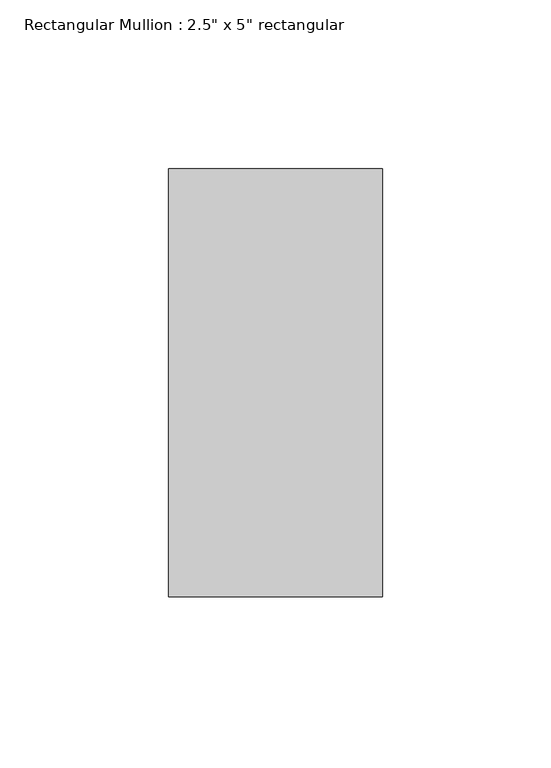
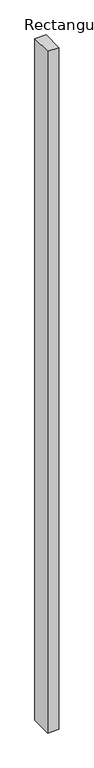
"""IFC4 building model written with IfcOpenShell, lengths in millimetres: member geometry."""

from ifc_helpers import new_model, si_unit, frame, origin, place, context, project, spatial, polyline, outline, extrude, source, transform, mapped, element, save


def member_d84c53df(model_context):
    return source(origin(), model_context, "Body", "SweptSolid", [
        extrude(outline(polyline([(0.0, 63.5), (0.0, -63.5), (-63.5, -63.5), (-63.5, 63.5), (0.0, 63.5)])), frame((0.0, 0.0, -4104.1288793), z_axis=(0.0, 0.0, 1.0), x_axis=(1.0, 0.0, 0.0)), (0.0, 0.0, 1.0), 4104.1288793),
    ])


if __name__ == "__main__":
    model = new_model("IFC4")
    model_context = context("Model", 3, world=origin())
    ifc_project = project(units=[si_unit("LENGTHUNIT", "METRE", prefix="MILLI")], contexts=[model_context])
    site = spatial("IfcSite", under=ifc_project)
    building = spatial("IfcBuilding", under=site)
    placement = place(None, origin())
    member_shape = member_d84c53df(model_context)
    element("IfcMember", 1, ObjectType="Rectangular Mullion : 2.5\" x 5\" rectangular", at=placement, inside=building, context=model_context, shape_type="MappedRepresentation", body=[
        mapped(member_shape, transform((0.0, 0.0, 0.0), x_axis=(1.0, 0.0, 0.0), y_axis=(0.0, 1.0, 0.0), z_axis=(0.0, 0.0, 1.0))),
    ])
    save(model, "model.ifc")

# Revit data of these elements
# Type "Rectangular Mullion : 2.5\" x 5\" rectangular"
#   built-in parameter 1007304 = 0.416667 (stored number, unit not read)
#   built-in parameter 1007301 = 0.104167 (stored number, unit not read)
#   built-in parameter 1007300 = 0.104167 (stored number, unit not read)
# Element 1 (IfcMember, "Rectangular Mullion : 2.5\" x 5\" rectangular")
#   Materials on its faces: "Aluminum"
# Materials
#   "Aluminum": class "Metal", colour RGB 247 247 247, transparency 0, Description = "Aluminum 6061", Cost = 0
